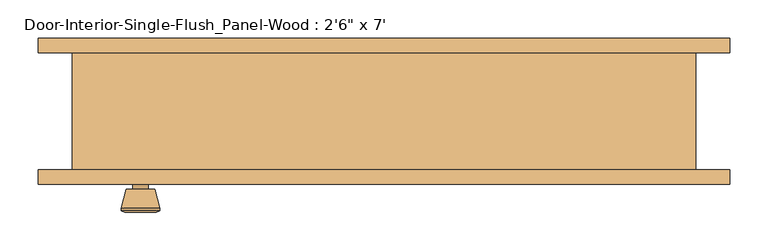
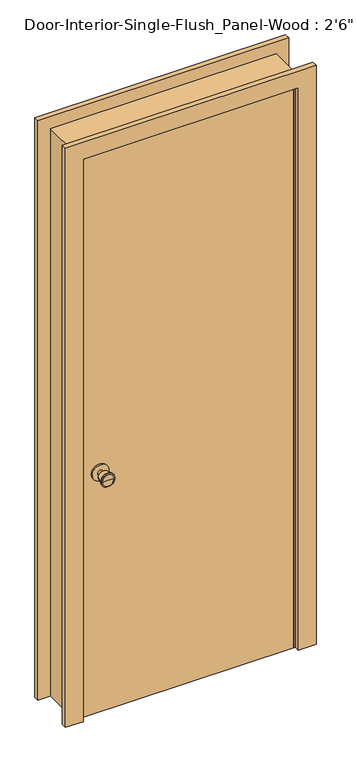
"""IFC4 building model written with IfcOpenShell, lengths in millimetres: door geometry."""

from ifc_helpers import new_model, si_unit, point, frame, frame_2d, origin, origin_with_axes, place, context, project, spatial, polyline, circle_curve, trimmed, segment, composite_curve, outline, extrude, faceted_brep, source, transform, mapped, element, save
from ifc_brep_helpers import plane_surface, cylinder_surface, revolved_surface, advanced_brep


def door_6764305a(model_context):
    return source(origin(), model_context, "Body", "SolidModel", [
        advanced_brep(
        [(-317.5, -32.1, 914.4), (-327.5, -32.1, 914.4), (-307.5, -32.1, 914.4), (-297.0241324, 16.9, 914.4), (-337.9758676, 16.9, 914.4), (-317.5, 16.9, 914.4), (-292.5, 15.0721319, 914.4), (-342.5, 15.0721319, 914.4), (-292.5, 11.6084537, 914.4), (-342.5, 11.6084537, 914.4), (-298.863764, -13.1, 914.4), (-336.136236, -13.1, 914.4), (-307.5, -13.1, 914.4), (-327.5, -13.1, 914.4)],
        [
            (0, 1),
            (1, 2, circle_curve(frame((-317.5, -32.1, 914.4), z_axis=(0.0, -1.0, 0.0), x_axis=(-1.0, 0.0, 0.0)), 10.0)),
            (2, 0),
            (2, 1, circle_curve(frame((-317.5, -32.1, 914.4), z_axis=(0.0, -1.0, 0.0), x_axis=(-1.0, 0.0, 0.0)), 10.0)),
            (3, 4, circle_curve(frame((-317.5, 16.9, 914.4), z_axis=(0.0, 1.0, 0.0), x_axis=(-1.0, 0.0, 0.0)), 20.4758676)),
            (4, 5),
            (5, 3),
            (4, 3, circle_curve(frame((-317.5, 16.9, 914.4), z_axis=(0.0, 1.0, 0.0), x_axis=(-1.0, 0.0, 0.0)), 20.4758676)),
            (6, 7, circle_curve(frame((-317.5, 15.0721319, 914.4), z_axis=(0.0, 1.0, 0.0), x_axis=(-1.0, 0.0, 0.0)), 25.0)),
            (7, 4),
            (3, 6),
            (7, 6, circle_curve(frame((-317.5, 15.0721319, 914.4), z_axis=(0.0, 1.0, 0.0), x_axis=(-1.0, 0.0, 0.0)), 25.0)),
            (8, 9, circle_curve(frame((-317.5, 11.6084537, 914.4), z_axis=(0.0, 1.0, 0.0), x_axis=(-1.0, 0.0, 0.0)), 25.0)),
            (9, 7),
            (6, 8),
            (9, 8, circle_curve(frame((-317.5, 11.6084537, 914.4), z_axis=(0.0, 1.0, 0.0), x_axis=(-1.0, 0.0, 0.0)), 25.0)),
            (10, 11, circle_curve(frame((-317.5, -13.1, 914.4), z_axis=(0.0, 1.0, 0.0), x_axis=(-1.0, 0.0, 0.0)), 18.636236)),
            (11, 9),
            (8, 10),
            (11, 10, circle_curve(frame((-317.5, -13.1, 914.4), z_axis=(0.0, 1.0, 0.0), x_axis=(-1.0, 0.0, 0.0)), 18.636236)),
            (12, 13, circle_curve(frame((-317.5, -13.1, 914.4), z_axis=(0.0, 1.0, 0.0), x_axis=(-1.0, 0.0, 0.0)), 10.0)),
            (13, 11),
            (10, 12),
            (13, 12, circle_curve(frame((-317.5, -13.1, 914.4), z_axis=(0.0, 1.0, 0.0), x_axis=(-1.0, 0.0, 0.0)), 10.0)),
            (1, 13),
            (12, 2),
        ],
        [
            plane_surface(frame((-317.5, -32.1, 914.4), z_axis=(0.0, -1.0, 0.0), x_axis=(-1.0, 0.0, 0.0))),
            plane_surface(frame((-317.5, 16.9, 914.4), z_axis=(0.0, 1.0, 0.0), x_axis=(-1.0, 0.0, 0.0))),
            revolved_surface(polyline([(-337.9758676, 16.9, 914.4), (-342.5, 15.0721319, 914.4)]), (-317.5, -32.1, 914.4), (0.0, -1.0, 0.0)),
            cylinder_surface(frame((-317.5, -32.1, 914.4), z_axis=(0.0, -1.0, 0.0), x_axis=(-1.0, 0.0, 0.0)), 25.0),
            revolved_surface(polyline([(-342.5, 11.6084537, 914.4), (-336.136236, -13.1, 914.4)]), (-317.5, -32.1, 914.4), (0.0, -1.0, 0.0)),
            plane_surface(frame((-317.5, -13.1, 914.4), z_axis=(0.0, -1.0, 0.0), x_axis=(-1.0, 0.0, 0.0))),
            cylinder_surface(frame((-317.5, -32.1, 914.4), z_axis=(0.0, -1.0, 0.0), x_axis=(-1.0, 0.0, 0.0)), 10.0),
        ],
        [
            (0, [[1, 2, 3]]),
            (0, [[-3, 4, -1]]),
            (1, [[5, 6, 7]]),
            (1, [[8, -7, -6]]),
            (2, [[9, 10, -5, 11]]),
            (2, [[12, -11, -8, -10]]),
            (3, [[13, 14, -9, 15]]),
            (3, [[16, -15, -12, -14]]),
            (4, [[17, 18, -13, 19]]),
            (4, [[20, -19, -16, -18]]),
            (5, [[21, 22, -17, 23]]),
            (5, [[24, -23, -20, -22]]),
            (6, [[-2, 25, -21, 26]]),
            (6, [[-4, -26, -24, -25]]),
        ],
    ),
        extrude(outline(composite_curve([segment(trimmed(circle_curve(frame_2d((914.4, -317.5)), 30.0), [point((914.4, -347.5))], [point((914.4, -287.5))], False, "CARTESIAN"), True, "CONTINUOUS"), segment(trimmed(circle_curve(frame_2d((914.4, -317.5)), 30.0), [point((914.4, -287.5))], [point((914.4, -347.5))], False, "CARTESIAN"), True, "CONTINUOUS")], self_intersect=False)), frame((0.0, -38.1, 0.0), z_axis=(0.0, 1.0, 0.0), x_axis=(0.0, 0.0, 1.0)), (0.0, 0.0, 1.0), 6.0),
        advanced_brep(
        [(-317.5, -79.025, 914.4), (-307.5, -79.025, 914.4), (-327.5, -79.025, 914.4), (-297.0241324, -128.025, 914.4), (-317.5, -128.025, 914.4), (-337.9758676, -128.025, 914.4), (-292.5, -126.1971319, 914.4), (-342.5, -126.1971319, 914.4), (-292.5, -122.7334537, 914.4), (-342.5, -122.7334537, 914.4), (-298.863764, -98.025, 914.4), (-336.136236, -98.025, 914.4), (-307.5, -98.025, 914.4), (-327.5, -98.025, 914.4)],
        [
            (0, 1),
            (1, 2, circle_curve(frame((-317.5, -79.025, 914.4), z_axis=(0.0, 1.0, 0.0), x_axis=(-1.0, 0.0, 0.0)), 10.0)),
            (2, 0),
            (2, 1, circle_curve(frame((-317.5, -79.025, 914.4), z_axis=(0.0, 1.0, 0.0), x_axis=(-1.0, 0.0, 0.0)), 10.0)),
            (3, 4),
            (4, 5),
            (5, 3, circle_curve(frame((-317.5, -128.025, 914.4), z_axis=(0.0, -1.0, 0.0), x_axis=(-1.0, 0.0, 0.0)), 20.4758676)),
            (3, 5, circle_curve(frame((-317.5, -128.025, 914.4), z_axis=(0.0, -1.0, 0.0), x_axis=(-1.0, 0.0, 0.0)), 20.4758676)),
            (6, 3),
            (5, 7),
            (7, 6, circle_curve(frame((-317.5, -126.1971319, 914.4), z_axis=(0.0, -1.0, 0.0), x_axis=(-1.0, 0.0, 0.0)), 25.0)),
            (6, 7, circle_curve(frame((-317.5, -126.1971319, 914.4), z_axis=(0.0, -1.0, 0.0), x_axis=(-1.0, 0.0, 0.0)), 25.0)),
            (8, 6),
            (7, 9),
            (9, 8, circle_curve(frame((-317.5, -122.7334537, 914.4), z_axis=(0.0, -1.0, 0.0), x_axis=(-1.0, 0.0, 0.0)), 25.0)),
            (8, 9, circle_curve(frame((-317.5, -122.7334537, 914.4), z_axis=(0.0, -1.0, 0.0), x_axis=(-1.0, 0.0, 0.0)), 25.0)),
            (10, 8),
            (9, 11),
            (11, 10, circle_curve(frame((-317.5, -98.025, 914.4), z_axis=(0.0, -1.0, 0.0), x_axis=(-1.0, 0.0, 0.0)), 18.636236)),
            (10, 11, circle_curve(frame((-317.5, -98.025, 914.4), z_axis=(0.0, -1.0, 0.0), x_axis=(-1.0, 0.0, 0.0)), 18.636236)),
            (12, 10),
            (11, 13),
            (13, 12, circle_curve(frame((-317.5, -98.025, 914.4), z_axis=(0.0, -1.0, 0.0), x_axis=(-1.0, 0.0, 0.0)), 10.0)),
            (12, 13, circle_curve(frame((-317.5, -98.025, 914.4), z_axis=(0.0, -1.0, 0.0), x_axis=(-1.0, 0.0, 0.0)), 10.0)),
            (1, 12),
            (13, 2),
        ],
        [
            plane_surface(frame((-317.5, -79.025, 914.4), z_axis=(0.0, 1.0, 0.0), x_axis=(-1.0, 0.0, 0.0))),
            plane_surface(frame((-317.5, -128.025, 914.4), z_axis=(0.0, -1.0, 0.0), x_axis=(-1.0, 0.0, 0.0))),
            revolved_surface(polyline([(-337.9758676, -128.025, 914.4), (-342.5, -126.1971319, 914.4)]), (-317.5, -79.025, 914.4), (0.0, 1.0, 0.0)),
            cylinder_surface(frame((-317.5, -79.025, 914.4), z_axis=(0.0, 1.0, 0.0), x_axis=(-1.0, 0.0, 0.0)), 25.0),
            revolved_surface(polyline([(-342.5, -122.7334537, 914.4), (-336.136236, -98.025, 914.4)]), (-317.5, -79.025, 914.4), (0.0, 1.0, 0.0)),
            plane_surface(frame((-317.5, -98.025, 914.4), z_axis=(0.0, 1.0, 0.0), x_axis=(-1.0, 0.0, 0.0))),
            cylinder_surface(frame((-317.5, -79.025, 914.4), z_axis=(0.0, 1.0, 0.0), x_axis=(-1.0, 0.0, 0.0)), 10.0),
        ],
        [
            (0, [[1, 2, 3]]),
            (0, [[-3, 4, -1]]),
            (1, [[5, 6, 7]]),
            (1, [[-6, -5, 8]]),
            (2, [[9, -7, 10, 11]]),
            (2, [[-10, -8, -9, 12]]),
            (3, [[13, -11, 14, 15]]),
            (3, [[-14, -12, -13, 16]]),
            (4, [[17, -15, 18, 19]]),
            (4, [[-18, -16, -17, 20]]),
            (5, [[21, -19, 22, 23]]),
            (5, [[-22, -20, -21, 24]]),
            (6, [[25, -23, 26, -2]]),
            (6, [[-26, -24, -25, -4]]),
        ],
    ),
        extrude(outline(composite_curve([segment(trimmed(circle_curve(frame_2d((914.4, -317.5)), 30.0), [point((914.4, -347.5))], [point((914.4, -287.5))], False, "CARTESIAN"), True, "CONTINUOUS"), segment(trimmed(circle_curve(frame_2d((914.4, -317.5)), 30.0), [point((914.4, -287.5))], [point((914.4, -347.5))], False, "CARTESIAN"), True, "CONTINUOUS")], self_intersect=False)), frame((0.0, -79.025, 0.0), z_axis=(0.0, 1.0, 0.0), x_axis=(0.0, 0.0, 1.0)), (0.0, 0.0, 1.0), 6.0),
        faceted_brep([(406.4, -73.025, 0.0), (381.0, -73.025, 0.0), (381.0, -38.1, 0.0), (368.3, -38.1, 0.0), (368.3, -3.175, 0.0), (381.0, -3.175, 0.0), (381.0, 79.375, 0.0), (406.4, 79.375, 0.0), (406.4, 79.375, 2159.0), (406.4, -73.025, 2159.0), (381.0, 79.375, 2133.6), (-381.0, 79.375, 2133.6), (-381.0, 79.375, 0.0), (-406.4, 79.375, 0.0), (-406.4, 79.375, 2159.0), (381.0, -3.175, 2133.6), (368.3, -3.175, 2120.9), (-368.3, -3.175, 2120.9), (-368.3, -3.175, 0.0), (-381.0, -3.175, 0.0), (-381.0, -3.175, 2133.6), (368.3, -38.1, 2120.9), (381.0, -38.1, 2133.6), (-381.0, -38.1, 2133.6), (-381.0, -38.1, 0.0), (-368.3, -38.1, 0.0), (-368.3, -38.1, 2120.9), (381.0, -73.025, 2133.6), (-406.4, -73.025, 2159.0), (-406.4, -73.025, 0.0), (-381.0, -73.025, 0.0), (-381.0, -73.025, 2133.6)], [[[0, 1, 2, 3, 4, 5, 6, 7]], [[7, 8, 9, 0]], [[6, 10, 11, 12, 13, 14, 8, 7]], [[5, 15, 10, 6]], [[4, 16, 17, 18, 19, 20, 15, 5]], [[3, 21, 16, 4]], [[2, 22, 23, 24, 25, 26, 21, 3]], [[1, 27, 22, 2]], [[0, 9, 28, 29, 30, 31, 27, 1]], [[8, 14, 28, 9]], [[15, 20, 11, 10]], [[21, 26, 17, 16]], [[27, 31, 23, 22]], [[29, 13, 12, 19, 18, 25, 24, 30]], [[14, 13, 29, 28]], [[20, 19, 12, 11]], [[26, 25, 18, 17]], [[31, 30, 24, 23]]]),
        extrude(outline(polyline([(381.0, -38.1), (381.0, -73.025), (-381.0, -73.025), (-381.0, -38.1), (381.0, -38.1)])), origin_with_axes(), (0.0, 0.0, 1.0), 2133.6),
        extrude(outline(polyline([(0.0, 450.85), (2203.45, 450.85), (2203.45, -450.85), (0.0, -450.85), (0.0, -387.35), (2139.95, -387.35), (2139.95, 387.35), (0.0, 387.35), (0.0, 450.85)])), frame((0.0, -92.075, 0.0), z_axis=(0.0, 1.0, 0.0), x_axis=(0.0, 0.0, 1.0)), (0.0, 0.0, 1.0), 19.05),
        extrude(outline(polyline([(0.0, 450.85), (2203.45, 450.85), (2203.45, -450.85), (0.0, -450.85), (0.0, -387.35), (2139.95, -387.35), (2139.95, 387.35), (0.0, 387.35), (0.0, 450.85)])), frame((0.0, 79.375, 0.0), z_axis=(0.0, 1.0, 0.0), x_axis=(0.0, 0.0, 1.0)), (0.0, 0.0, 1.0), 19.05),
    ])


if __name__ == "__main__":
    model = new_model("IFC4")
    model_context = context("Model", 3, world=origin())
    ifc_project = project(units=[si_unit("LENGTHUNIT", "METRE", prefix="MILLI")], contexts=[model_context])
    site = spatial("IfcSite", under=ifc_project)
    building = spatial("IfcBuilding", under=site)
    placement = place(None, origin())
    door_shape = door_6764305a(model_context)
    element("IfcDoor", 1, ObjectType="Door-Interior-Single-Flush_Panel-Wood : 2'6\" x 7'", at=placement, inside=building, context=model_context, shape_type="MappedRepresentation", body=[
        mapped(door_shape, transform((0.0, 0.0, 0.0), x_axis=(1.0, 0.0, 0.0), y_axis=(0.0, 1.0, 0.0), z_axis=(0.0, 0.0, 1.0))),
    ])
    save(model, "model.ifc")

# Revit data of these elements
# Type "Door-Interior-Single-Flush_Panel-Wood : 2'6\" x 7'"
#   Type Mark = "13"
#   Assembly Code = "C1020300"
#   Analytic Construction = "Wooden"
#   Thickness = 0' - 1 3/8"
#   Thermal Resistance (R) = 2.5876 (h·ft²·°F)/BTU
#   Swing Angle [instance default] = 90.00°
#   Rough Width = 2' - 8"
#   Rough Height = 7' - 1"
#   Height = 7' - 0"
#   Width = 2' - 6"
#   Heat Transfer Coefficient (U) = 0.3865 BTU/(h·ft²·°F)
#   Trim Material = Cherry
#   Panel Material = Cherry
#   Frame Material = Cherry
#   Door Handle Material = Aluminum
#   Visual Light Transmittance = 0
#   Solar Heat Gain Coefficient = 0
#   Wall Closure = (empty or 0)
#   Function = (empty or 0)
# Element 1 (IfcDoor, "Door-Interior-Single-Flush_Panel-Wood : 2'6\" x 7'")
#   Materials on its faces: "Cherry", "Aluminum"
# Materials
#   "Cherry": class "Wood", colour RGB 226 177 128, transparency 0, Description = "Prunus Serotina", Cost = 0
#   "Aluminum": class "Metal", colour RGB 247 247 247, transparency 0, Description = "Aluminum 6061", Cost = 0
